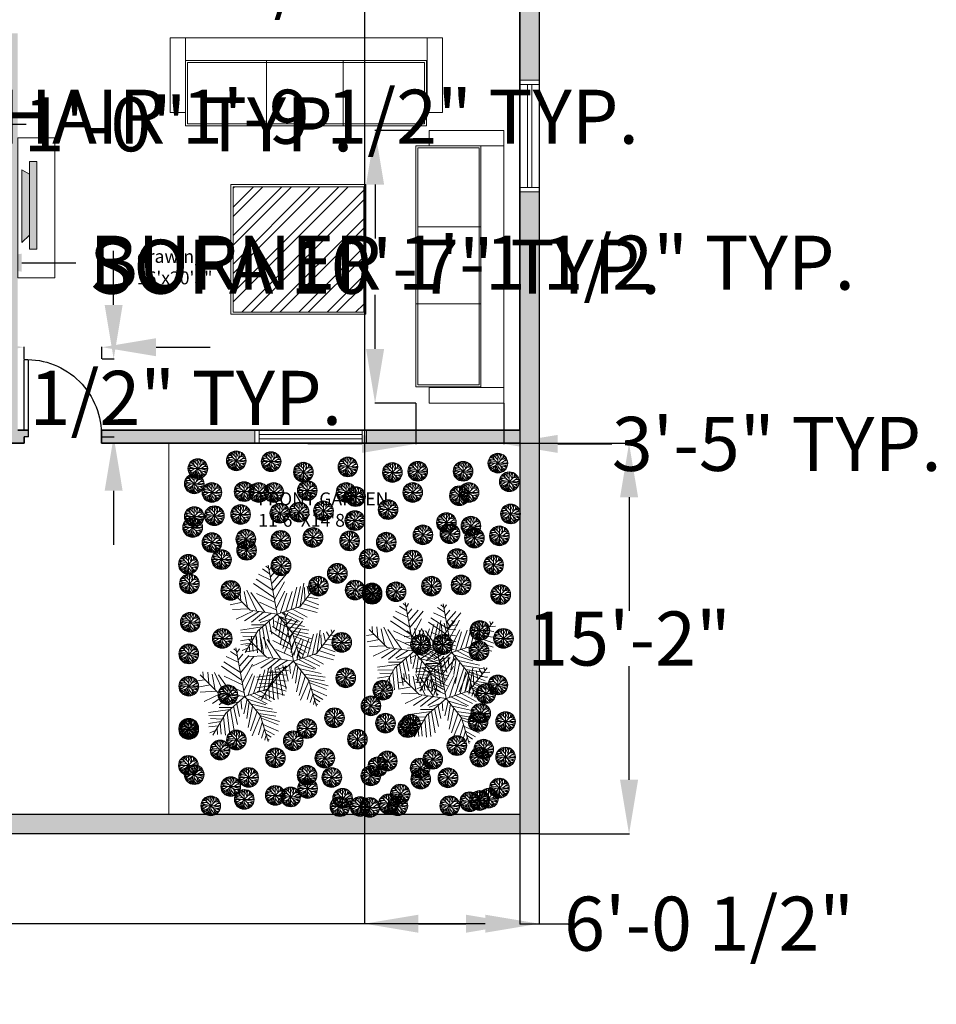
# Model space of a CAD drawing. Units: inches. Extents: x 23 to 3024, y 4 to 1405.
# Tile 4 of 7: x 2558 to 2985, y 497 to 955. Entities that reach past the tile are written whole.
import ezdxf

# ---------------------------------------------------------------- set-up
doc = ezdxf.new("R2010")
doc.units = ezdxf.units.IN
doc.header["$MEASUREMENT"] = 0
for name, color, linetype, lineweight in [('A-ANNO-DIMS', 2, 'Continuous', 18), ('A-DOOR', 4, 'Continuous', 25), ('A-EQPM', 8, 'Continuous', 18), ('A-EQPM-PATT', 7, 'Continuous', 13), ('A-WALL', 7, 'Continuous', 35), ('A-WALL-PATT', 189, 'Continuous', 13), ('C-PROP', 7, 'Continuous', 30), ('L-HRDS', 8, 'Continuous', 18), ('L-PLNT', 114, 'Continuous', 13)]:
    doc.layers.add(name, color=color, linetype=linetype, lineweight=lineweight)
for name, color, linetype, lineweight, true_color in [('A-AREA-IDEN', 30, 'Continuous', 18, 0xf8991e), ('A-FURN', 141, 'Continuous', 18, 0xadddf7), ('A-FURN-PATT', 215, 'Continuous', 13, 0xa953a0), ('A-GLAZ', 30, 'Continuous', 18, 0xf26722)]:
    doc.layers.add(name, color=color, linetype=linetype, lineweight=lineweight, true_color=true_color)
doc.styles.get("Standard").update_dxf_attribs({"font": 'arial.ttf'})
doc.dimstyles.get("Standard").update_dxf_attribs({"dimtxt": 25.18, "dimasz": 25.18, "dimexe": 0.18, "dimexo": 0.0625, "dimgap": 0.09, "dimtad": 0, "dimtih": 1, "dimtoh": 1, "dimdec": 0, "dimrnd": 10, "dimzin": 0, "dimdsep": 46, "dimlunit": 3, "dimtxsty": 'Standard', "dimcen": 0.09, "dimadec": 0, "dimazin": 0, "dimtfac": 1, "dimtdec": 0, "dimtofl": 0, "dimtmove": 0, "dimatfit": 3, "dimfxl": 1, "dimtolj": 1, "dimtzin": 0, "dimarcsym": 0})

# ---------------------------------------------------------------- blocks, each defined once
blk = doc.blocks.new('Tree - deciduous plan')
for p, q in [((2.426, 54.9406), (-1.4472, 59.9056)), ((0, 59.9996), (0, -60)), ((-59.7219, 2.8025), (-12.0106, 12.0565)), ((-32.2571, 20.6333), (-59.1937, 9.348)), ((-58.6656, 12.7336), (-35.9543, 7.5424)), ((-57.081, 17.9248), (-47.0458, 14.7649)), ((-56.0247, 20.859), (-20.8134, 20.859)), ((-54.7923, 24.4702), (-47.75, 21.0847)), ((-54.6162, -24.7335), (-20.2853, 0.0941)), ((-53.2078, 27.4044), (-40.1797, 20.859)), ((-49.8627, 32.8214), (-32.7853, 32.8214)), ((-45.8134, 38.2383), (-40.5318, 33.0471)), ((-43.8768, 36.4326), (-44.405, 40.2696)), ((42, 42), (-42, -42)), ((42, -42), (-42, 42)), ((-40.1797, 44.558), (-36.4825, 43.2038)), ((-37.0107, 47.0408), (-35.25, 35.5298)), ((-32.6092, 50.4264), (-23.2782, 23.5674)), ((-31.2008, 51.1035), (-0.2149, 20.1818)), ((-26.4472, 46.5894), (-26.2712, 53.8116)), ((-22.0458, 42.0753), (-16.5881, 57.6486)), ((-21.1656, 55.8436), (-0.0388, 45.0094)), ((-12.5388, 54.9406), (-7.9613, 59.4546)), ((-12.3627, 32.1443), (-12.5388, 58.7776)), ((-5.3205, 59.6806), (16.5105, 16.7963)), ((0.4894, 48.6208), (3.6584, 59.6806)), ((18.2711, 35.5298), (5.419, 59.6806)), ((9.8203, 51.5549), (12.8133, 58.5516)), ((19.6795, 19.5047), (16.3344, 57.6486)), ((17.0387, 51.1035), (23.2006, 55.1666)), ((17.7429, 43.6552), (25.4894, 54.2636)), ((54.3626, 25.3731), (20.9119, 0.3198)), ((23.3767, 23.3417), (53.3063, 27.4044)), ((29.3626, -6.6771), (59.4682, 7.091)), ((31.6513, 50.8778), (30.2429, 30.5643)), ((31.1232, 42.5267), (35.8767, 48.1693)), ((36.2288, 25.1474), (48.9049, 35.0784)), ((37.1091, 37.1098), (46.6161, 37.5612)), ((38.5175, 13.4107), (58.2359, 13.6364)), ((-60, 0), (60, 0)), ((-59.7219, -4.8714), (-54.2641, -6.6771)), ((-45.2853, -0.1316), (-59.0177, -10.0627)), ((-58.4895, -12.3197), (-36.4825, -11.6426)), ((-57.081, -18.4138), (-45.2853, -17.9624)), ((-52.6797, -18.188), (-55.4966, -22.0251)), ((-53.2078, -27.442), (-16.7641, -16.6081)), ((-38.9472, -29.0219), (-51.4472, -30.6018)), ((-47.2219, -19.3166), (-50.2148, -26.3135)), ((-46.5177, -30.1504), (-49.5106, -33.536)), ((-32.4331, -32.4075), (-48.1021, -35.5674)), ((-43.7008, -34.6645), (-46.6937, -37.373)), ((-35.9543, -22.4765), (-44.0529, -40.5329)), ((-24.6867, -37.8244), (-38.7712, -45.7241)), ((-26.2712, -43.9185), (-34.7219, -48.6583)), ((-19.9331, -20.2194), (-28.5599, -52.721)), ((-14.6515, -36.2445), (-27.6797, -52.9467)), ((-14.6515, -47.3041), (-25.0388, -54.3009)), ((-21.5177, -45.4984), (-19.9331, -56.1065)), ((-14.8275, -15.0282), (-14.6515, -57.6865)), ((-14.6515, -32.1818), (-3.912, -59.4922)), ((-8.4895, -47.5298), (-11.4825, -58.5893)), ((-10.074, -10.0627), (-2.5036, -59.7178)), ((-6.3768, -52.721), (-9.3698, -58.815)), ((-6.2008, -36.2445), (17.919, -57.0094)), ((-0.0388, -19.0909), (25.8415, -53.8495)), ((8.4119, -53.1724), (3.8344, -59.4922)), ((5.9471, -46.6269), (10.5246, -58.5893)), ((9.2922, -9.1598), (59.6443, -2.8401)), ((18.6232, -18.6394), (26.7218, -53.3981)), ((18.7992, -18.6394), (57.3556, -17.2853)), ((22.8485, -36.4702), (35.3485, -48.4326)), ((24.7852, -44.8213), (23.0246, -54.978)), ((26.3697, -18.4138), (58.9401, -9.8369)), ((30.419, -30.1504), (32.3556, -50.0125)), ((31.4753, -31.279), (49.6091, -33.3103)), ((38.1654, -18.188), (52.426, -29.0219)), ((41.5105, -32.6332), (46.088, -38.0501)), ((45.9119, -24.0564), (55.595, -22.2508))]:
    blk.add_line(p, q)
blk.add_circle((0, 0), 60)
blk = doc.blocks.new('*U8')
for p, q in [((-7.288, 39.707), (-21.778, 46.673)), ((-8.737, 47.138), (-17.069, 52.711)), ((-10.186, 53.64), (-13.084, 55.962)), ((0, 0), (-10.5, 57)), ((-9.099, 51.782), (-6.563, 55.962)), ((-7.65, 43.423), (-2.578, 49.46)), ((-5.839, 35.992), (4.667, 48.067)), ((-5.114, 27.632), (10.463, 46.673)), ((-3.665, 19.273), (-27.574, 35.527)), ((-5.114, 28.097), (-24.676, 40.636)), ((-2.941, 16.486), (8.652, 37.85)), ((27, 9), (48, 36)), ((27.127, 9.056), (31.112, 35.992)), ((44.153, 36.456), (45.239, 32.741)), ((-31.5, 4.5), (-52.5, 25.5)), ((-48.585, 21.131), (-49.309, 29.026)), ((-43.513, 28.561), (-42.427, 15.558)), ((-38.442, 26.239), (-34.819, 7.663)), ((-35.544, 28.097), (-24.314, 3.947)), ((-14.533, 2.09), (-30.834, 25.31)), ((-24.314, 23.917), (-2.941, 13.7)), ((-1.129, 6.734), (9.014, 26.704)), ((3.942, 1.625), (11.187, 24.381)), ((10.101, 3.483), (17.708, 26.239)), ((16.259, 5.805), (23.142, 31.348)), ((22.055, 7.198), (27.489, 32.277)), ((31.836, 30.883), (32.561, 16.486)), ((35.096, 32.741), (37.27, 22.524)), ((38.719, 34.134), (41.979, 28.561)), ((40.53, 25.775), (48.862, 24.846)), ((43.791, 29.954), (51.036, 30.883)), ((-47.498, 19.737), (-55.83, 18.344)), ((-40.615, 13.7), (-55.105, 10.913)), ((-20.691, 13.7), (-1.129, 4.876)), ((29.662, 12.307), (48.137, 6.269)), ((33.285, 16.486), (48.862, 10.913)), ((36.183, 19.737), (48.137, 17.88)), ((-33.37, 6.269), (-52.207, 5.34)), ((-28.299, 3.483), (-47.86, -5.805)), ((-21.416, 3.018), (-38.079, -8.128)), ((0, 0), (-31.5, 4.5)), ((-15.982, 2.09), (-30.11, -9.521)), ((0, 0), (-22.5, -19.5)), ((-6.563, 1.161), (-21.416, -8.128)), ((0, 0), (27, 9)), ((0, 0), (18, -22.5)), ((6.478, 1.625), (26.04, -8.592)), ((11.187, 3.483), (30.749, -5.805)), ((18.07, 5.805), (35.096, -3.483)), ((24.229, 7.663), (46.688, 1.625)), ((-6.563, -5.805), (-19.967, -9.985)), ((-13.446, -11.378), (-8.737, -32.741)), ((-9.461, -8.592), (-6.201, -23.453)), ((-4.752, -3.483), (-3.665, -14.629)), ((2.493, -3.019), (-1.491, -20.202)), ((1.769, -2.555), (24.229, -9.521)), ((5.029, -6.27), (2.131, -25.775)), ((9.014, -11.378), (3.58, -35.992)), ((7.565, -9.056), (32.198, -14.629)), ((-17.431, -15.094), (-42.789, -18.809)), ((-24.314, -21.596), (-42.427, -22.06)), ((-22.5, -19.5), (-37.5, -45)), ((-15.257, -12.772), (-30.11, -12.772)), ((-20.691, -18.345), (-17.793, -44.352)), ((-17.069, -15.094), (-12.721, -40.172)), ((14.085, -16.951), (6.478, -40.172)), ((18.07, -22.524), (8.289, -45.745)), ((12.274, -15.094), (36.907, -18.809)), ((16.259, -19.738), (36.183, -22.989)), ((18, -22.5), (27, -52.5)), ((18.433, -22.524), (40.53, -29.026)), ((-28.299, -29.026), (-42.789, -31.348)), ((-30.834, -34.135), (-42.427, -35.528)), ((-26.849, -26.24), (-40.253, -25.775)), ((-29.023, -30.884), (-27.936, -43.887)), ((-25.038, -23.918), (-22.865, -45.281)), ((20.244, -30.419), (15.897, -44.816)), ((19.157, -25.311), (38.719, -33.206)), ((21.331, -32.741), (39.081, -40.636)), ((-34.457, -39.708), (-40.978, -42.494)), ((-32.646, -36.921), (-31.921, -44.352)), ((22.78, -37.85), (19.519, -48.532)), ((22.78, -38.314), (34.372, -44.816)), ((24.591, -45.745), (23.142, -50.854)), ((24.591, -43.423), (30.749, -47.603)), ((26.764, -49.925), (28.213, -50.854))]:
    blk.add_line(p, q)
blk = doc.blocks.new('DOOR-SWING-36IN')
for p, q in [((-1, -1), (-1, 35)), ((1, 2), (1, 35)), ((-1, -1), (1, -1))]:
    blk.add_line(p, q)
blk.add_arc((0, 0), 35.01, 88.3634, 181.6366)
blk = doc.blocks.new('WINDOW-48IN')
for p, q in [((9, 52), (0, 52)), ((9, 50), (0, 50)), ((3.5, 2), (3.5, 50)), ((5.5, 2), (5.5, 50)), ((9, 2), (0, 2)), ((9, 0), (0, 0))]:
    blk.add_line(p, q)
blk = doc.blocks.new('SOFA-THREE-SEAT')
for p, q in [((44.91, 30.29), (44.91, 0.86)), ((80.71, 30.29), (80.71, 0))]:
    blk.add_line(p, q)
for points in [[(7.2, 40.92), (0, 40.92), (0, 6.21), (7.2, 6.21)], [(7.2, 30.29), (119.76, 30.29), (119.76, 40.92), (7.2, 40.92)], [(126.96, 40.92), (119.76, 40.92), (119.76, 6.21), (126.96, 6.21)], [(7.2, 30.29), (119.4, 30.29), (119.4, 0), (7.2, 0)], [(8.06, 29.42), (118.53, 29.42), (118.53, 0.86), (8.06, 0.86)]]:
    blk.add_lwpolyline(points, close=True)
blk = doc.blocks.new('*D21')
at = {"layer": 'A-ANNO-DIMS', "color": 0, "lineweight": -2, "transparency": 16777216}
for p, q in [((2449.18, 913.2), (2449.18, 909.84)), ((2470.74, 913.2), (2470.74, 909.84)), ((2424, 910.02), (2398.82, 910.02)), ((2495.92, 910.02), (2521.1, 910.02))]:
    blk.add_line(p, q, dxfattribs=at)
at = {"layer": 'A-ANNO-DIMS', "color": 0, "transparency": 16777216}
for points in [[(2424, 914.22), (2424, 905.83), (2449.18, 910.02)], [(2495.92, 914.22), (2495.92, 905.83), (2470.74, 910.02)]]:
    blk.add_solid(points, dxfattribs=at)
at = {"layer": 'Defpoints', "color": 0, "transparency": 16777216}
for p in [(2449.18, 913.26), (2470.74, 913.26), (2470.74, 910.02)]:
    blk.add_point(p, dxfattribs=at)
at = {"layer": 'A-ANNO-DIMS', "color": 0, "transparency": 16777216, "insert": (2686.74, 910.02), "char_height": 25.18, "attachment_point": 5}
blk.add_mtext('\\A1;CHAIR 1\'-9 1/2" TYP.', dxfattribs=at)
blk = doc.blocks.new('*D22')
at = {"layer": 'A-ANNO-DIMS', "color": 0, "lineweight": -2, "transparency": 16777216}
for p, q in [((2473.98, 956.88), (2473.98, 982.06)), ((2473.98, 982.06), (2499.16, 982.06)), ((2470.81, 931.7), (2474.16, 931.7)), ((2470.81, 913.26), (2474.16, 913.26)), ((2473.98, 888.08), (2473.98, 862.9))]:
    blk.add_line(p, q, dxfattribs=at)
at = {"layer": 'A-ANNO-DIMS', "color": 0, "transparency": 16777216}
for points in [[(2469.78, 956.88), (2478.17, 956.88), (2473.98, 931.7)], [(2469.78, 888.08), (2478.17, 888.08), (2473.98, 913.26)]]:
    blk.add_solid(points, dxfattribs=at)
at = {"layer": 'Defpoints', "color": 0, "transparency": 16777216}
for p in [(2470.74, 931.7), (2473.98, 931.7), (2470.74, 913.26)]:
    blk.add_point(p, dxfattribs=at)
at = {"layer": 'A-ANNO-DIMS', "color": 0, "transparency": 16777216, "insert": (2604.14, 982.06), "char_height": 25.18, "attachment_point": 5}
blk.add_mtext('\\A1;1\'-6 1/2" TYP.', dxfattribs=at)
blk = doc.blocks.new('*D23')
at = {"layer": 'A-ANNO-DIMS', "color": 0, "lineweight": -2, "transparency": 16777216}
for p, q in [((2560.45, 797.26), (2560.45, 802.82)), ((2596.72, 797.26), (2596.72, 802.82)), ((2535.27, 802.64), (2510.09, 802.64)), ((2621.9, 802.64), (2647.08, 802.64))]:
    blk.add_line(p, q, dxfattribs=at)
at = {"layer": 'A-ANNO-DIMS', "color": 0, "transparency": 16777216}
for points in [[(2535.27, 806.84), (2535.27, 798.45), (2560.45, 802.64)], [(2621.9, 806.84), (2621.9, 798.45), (2596.72, 802.64)]]:
    blk.add_solid(points, dxfattribs=at)
at = {"layer": 'Defpoints', "color": 0, "transparency": 16777216}
for p in [(2560.45, 802.64), (2560.45, 797.2), (2596.72, 797.2)]:
    blk.add_point(p, dxfattribs=at)
at = {"layer": 'A-ANNO-DIMS', "color": 0, "transparency": 16777216, "insert": (2346.9, 802.64), "char_height": 25.18, "attachment_point": 5}
blk.add_mtext('\\A1;DOOR 3\'-0 1/2" TYP.', dxfattribs=at)
blk = doc.blocks.new('*D24')
at = {"layer": 'A-ANNO-DIMS', "color": 0, "lineweight": -2, "transparency": 16777216}
for p, q in [((2602.17, 822.38), (2602.17, 847.56)), ((2596.79, 797.2), (2602.35, 797.2)), ((2596.79, 760.93), (2602.35, 760.93)), ((2602.17, 735.75), (2602.17, 710.57))]:
    blk.add_line(p, q, dxfattribs=at)
at = {"layer": 'A-ANNO-DIMS', "color": 0, "transparency": 16777216}
for points in [[(2597.97, 822.38), (2606.36, 822.38), (2602.17, 797.2)], [(2597.97, 735.75), (2606.36, 735.75), (2602.17, 760.93)]]:
    blk.add_solid(points, dxfattribs=at)
at = {"layer": 'Defpoints', "color": 0, "transparency": 16777216}
for p in [(2596.72, 797.2), (2602.17, 797.2), (2596.72, 760.93)]:
    blk.add_point(p, dxfattribs=at)
at = {"layer": 'A-ANNO-DIMS', "color": 0, "transparency": 16777216, "insert": (2602.17, 779.06), "char_height": 25.18, "attachment_point": 5}
blk.add_mtext('\\A1;3\'-0 1/2" TYP.', dxfattribs=at)
blk = doc.blocks.new('*D31')
at = {"layer": 'A-ANNO-DIMS', "color": 0, "lineweight": -2, "transparency": 16777216}
for p, q in [((2742.95, 903.61), (2723.79, 903.61)), ((2723.97, 878.43), (2723.97, 853.25)), ((2723.97, 801.83), (2723.97, 827.01)), ((2742.95, 776.65), (2723.79, 776.65))]:
    blk.add_line(p, q, dxfattribs=at)
at = {"layer": 'A-ANNO-DIMS', "color": 0, "transparency": 16777216}
for points in [[(2719.77, 878.43), (2728.17, 878.43), (2723.97, 903.61)], [(2719.77, 801.83), (2728.17, 801.83), (2723.97, 776.65)]]:
    blk.add_solid(points, dxfattribs=at)
at = {"layer": 'Defpoints', "color": 0, "transparency": 16777216}
for p in [(2743.01, 903.61), (2723.97, 776.65), (2743.01, 776.65)]:
    blk.add_point(p, dxfattribs=at)
at = {"layer": 'A-ANNO-DIMS', "color": 0, "transparency": 16777216, "insert": (2723.97, 840.13), "char_height": 25.18, "attachment_point": 5}
blk.add_mtext('\\A1;SOFA 10\'-7" TYP.', dxfattribs=at)
blk = doc.blocks.new('*D32')
at = {"layer": 'A-ANNO-DIMS', "color": 0, "lineweight": -2, "transparency": 16777216}
for p, q in [((2743.01, 776.59), (2743.01, 757.43)), ((2783.93, 776.59), (2783.93, 757.43)), ((2717.83, 757.61), (2692.65, 757.61)), ((2809.11, 757.61), (2834.29, 757.61))]:
    blk.add_line(p, q, dxfattribs=at)
at = {"layer": 'A-ANNO-DIMS', "color": 0, "transparency": 16777216}
for points in [[(2717.83, 761.8), (2717.83, 753.41), (2743.01, 757.61)], [(2809.11, 761.8), (2809.11, 753.41), (2783.93, 757.61)]]:
    blk.add_solid(points, dxfattribs=at)
at = {"layer": 'Defpoints', "color": 0, "transparency": 16777216}
for p in [(2743.01, 776.65), (2783.93, 776.65), (2783.93, 757.61)]:
    blk.add_point(p, dxfattribs=at)
at = {"layer": 'A-ANNO-DIMS', "color": 0, "transparency": 16777216, "insert": (2911.12, 757.61), "char_height": 25.18, "attachment_point": 5}
blk.add_mtext('\\A1;3\'-5" TYP.', dxfattribs=at)
blk = doc.blocks.new('*D33')
at = {"layer": 'A-ANNO-DIMS', "color": 0, "lineweight": -2, "transparency": 16777216}
for p, q in [((2495.35, 842.02), (2470.17, 842.02)), ((2520.53, 844), (2520.53, 841.84)), ((2534.13, 844), (2534.13, 841.84)), ((2559.31, 842.02), (2584.49, 842.02))]:
    blk.add_line(p, q, dxfattribs=at)
at = {"layer": 'A-ANNO-DIMS', "color": 0, "transparency": 16777216}
for points in [[(2495.35, 846.22), (2495.35, 837.83), (2520.53, 842.02)], [(2559.31, 846.22), (2559.31, 837.83), (2534.13, 842.02)]]:
    blk.add_solid(points, dxfattribs=at)
at = {"layer": 'Defpoints', "color": 0, "transparency": 16777216}
for p in [(2520.53, 844.06), (2534.13, 844.06), (2534.13, 842.02)]:
    blk.add_point(p, dxfattribs=at)
at = {"layer": 'A-ANNO-DIMS', "color": 0, "transparency": 16777216, "insert": (2769.25, 842.02), "char_height": 25.18, "attachment_point": 5}
blk.add_mtext('\\A1;BURNER 1\'-1 1/2" TYP.', dxfattribs=at)
blk = doc.blocks.new('*D34')
at = {"layer": 'A-ANNO-DIMS', "color": 0, "lineweight": -2, "transparency": 16777216}
for p, q in [((2536.16, 881.33), (2536.16, 906.51)), ((2536.16, 906.51), (2561.34, 906.51)), ((2534.19, 856.15), (2536.34, 856.15)), ((2534.19, 844.06), (2536.34, 844.06)), ((2536.16, 818.88), (2536.16, 793.7))]:
    blk.add_line(p, q, dxfattribs=at)
at = {"layer": 'A-ANNO-DIMS', "color": 0, "transparency": 16777216}
for points in [[(2531.97, 881.33), (2540.36, 881.33), (2536.16, 856.15)], [(2531.97, 818.88), (2540.36, 818.88), (2536.16, 844.06)]]:
    blk.add_solid(points, dxfattribs=at)
at = {"layer": 'Defpoints', "color": 0, "transparency": 16777216}
for p in [(2534.13, 856.15), (2536.16, 856.15), (2534.13, 844.06)]:
    blk.add_point(p, dxfattribs=at)
at = {"layer": 'A-ANNO-DIMS', "color": 0, "transparency": 16777216, "insert": (2636.99, 906.51), "char_height": 25.18, "attachment_point": 5}
blk.add_mtext('\\A1;1\'-0" TYP.', dxfattribs=at)
blk = doc.blocks.new('*D35')
at = {"layer": 'A-ANNO-DIMS', "color": 0, "lineweight": -2, "transparency": 16777216}
for p, q in [((2272.06, 973.9), (2246.88, 973.9)), ((2297.24, 975.85), (2297.24, 973.72)), ((2310.67, 975.85), (2310.67, 973.72)), ((2335.85, 973.9), (2361.03, 973.9))]:
    blk.add_line(p, q, dxfattribs=at)
at = {"layer": 'A-ANNO-DIMS', "color": 0, "transparency": 16777216}
for points in [[(2272.06, 978.09), (2272.06, 969.7), (2297.24, 973.9)], [(2335.85, 978.09), (2335.85, 969.7), (2310.67, 973.9)]]:
    blk.add_solid(points, dxfattribs=at)
at = {"layer": 'Defpoints', "color": 0, "transparency": 16777216}
for p in [(2297.24, 975.91), (2310.67, 975.91), (2310.67, 973.9)]:
    blk.add_point(p, dxfattribs=at)
at = {"layer": 'A-ANNO-DIMS', "color": 0, "transparency": 16777216, "insert": (2585.8, 973.9), "char_height": 25.18, "attachment_point": 5}
blk.add_mtext('\\A1;NIGHTSTAND 1\'-1 1/2" TYP.', dxfattribs=at)
blk = doc.blocks.new('*D41')
at = {"layer": 'A-ANNO-DIMS', "color": 0, "lineweight": -2, "transparency": 16777216}
for p, q in [((2160.45, 575.86), (2160.45, 533.9)), ((2800.45, 575.86), (2800.45, 533.9)), ((2185.63, 534.08), (2437.11, 534.08)), ((2775.27, 534.08), (2523.79, 534.08))]:
    blk.add_line(p, q, dxfattribs=at)
at = {"layer": 'A-ANNO-DIMS', "color": 0, "transparency": 16777216}
for points in [[(2185.63, 538.27), (2185.63, 529.88), (2160.45, 534.08)], [(2775.27, 538.27), (2775.27, 529.88), (2800.45, 534.08)]]:
    blk.add_solid(points, dxfattribs=at)
at = {"layer": 'Defpoints', "color": 0, "transparency": 16777216}
for p in [(2160.45, 575.93), (2800.45, 575.93), (2800.45, 534.08)]:
    blk.add_point(p, dxfattribs=at)
at = {"layer": 'A-ANNO-DIMS', "color": 0, "transparency": 16777216, "insert": (2480.45, 534.08), "char_height": 25.18, "attachment_point": 5}
blk.add_mtext('\\A1;53\'-4"', dxfattribs=at)
blk = doc.blocks.new('*D42')
at = {"layer": 'A-ANNO-DIMS', "color": 0, "lineweight": -2, "transparency": 16777216}
for p, q in [((2791.51, 757.93), (2842.48, 757.93)), ((2842.3, 732.75), (2842.3, 679.87)), ((2842.3, 601.11), (2842.3, 653.98)), ((2800.51, 575.93), (2842.48, 575.93))]:
    blk.add_line(p, q, dxfattribs=at)
at = {"layer": 'A-ANNO-DIMS', "color": 0, "transparency": 16777216}
for points in [[(2838.1, 732.75), (2846.5, 732.75), (2842.3, 757.93)], [(2838.1, 601.11), (2846.5, 601.11), (2842.3, 575.93)]]:
    blk.add_solid(points, dxfattribs=at)
at = {"layer": 'Defpoints', "color": 0, "transparency": 16777216}
for p in [(2791.45, 757.93), (2842.3, 757.93), (2800.45, 575.93)]:
    blk.add_point(p, dxfattribs=at)
at = {"layer": 'A-ANNO-DIMS', "color": 0, "transparency": 16777216, "insert": (2842.3, 666.93), "char_height": 25.18, "attachment_point": 5}
blk.add_mtext('\\A1;15\'-2"', dxfattribs=at)
blk = doc.blocks.new('*D45')
at = {"layer": 'A-ANNO-DIMS', "color": 0, "lineweight": -2, "transparency": 16777216}
for p, q in [((2719, 988.72), (2719, 533.9)), ((2791.45, 988.72), (2791.45, 533.9)), ((2744.18, 534.08), (2766.27, 534.08)), ((2791.45, 534.08), (2816.63, 534.08))]:
    blk.add_line(p, q, dxfattribs=at)
at = {"layer": 'A-ANNO-DIMS', "color": 0, "transparency": 16777216}
for points in [[(2744.18, 538.27), (2744.18, 529.88), (2719, 534.08)], [(2766.27, 538.27), (2766.27, 529.88), (2791.45, 534.08)]]:
    blk.add_solid(points, dxfattribs=at)
at = {"layer": 'Defpoints', "color": 0, "transparency": 16777216}
for p in [(2719, 988.78), (2791.45, 988.78), (2791.45, 534.08)]:
    blk.add_point(p, dxfattribs=at)
at = {"layer": 'A-ANNO-DIMS', "color": 0, "transparency": 16777216, "insert": (2879.59, 534.08), "char_height": 25.18, "attachment_point": 5}
blk.add_mtext('\\A1;6\'-0 1/2"', dxfattribs=at)

msp = doc.modelspace()

# ---------------------------------------------------------------- hatches: boundary and pattern name
at = {"layer": 'A-EQPM-PATT'}
h = msp.add_hatch(color=256, dxfattribs=at)
h.dxf.hatch_style = 1
h.paths.add_polyline_path([(2566.39, 889.19), (2562.89, 889.19), (2562.89, 848.35), (2566.39, 848.35)])
h.paths.add_polyline_path([(2562.89, 883.28), (2559.32, 885.34), (2559.32, 851.44), (2562.89, 854.81)])
h.paths.add_polyline_path([(2370.36, 1159.16), (2369.43, 1157.81), (2369.43, 1135.58), (2370.36, 1134.43)])
h.paths.add_polyline_path([(2369.43, 1162.31), (2367.73, 1162.31), (2367.73, 1131.3), (2369.43, 1131.3)])
h.paths.add_polyline_path([(2381.34, 1160.62), (2379.7, 1162.16), (2380.08, 1134.79), (2381.34, 1136.43)])
h.paths.add_polyline_path([(2383.55, 1164.18), (2381.34, 1164.18), (2381.34, 1130.16), (2383.55, 1130.16)])
at = {"layer": 'A-FURN-PATT'}
h = msp.add_hatch(dxfattribs=at)
h.set_pattern_fill('ANSI32', color=256, scale=25)
h.paths.add_polyline_path([(2718.66, 877.42), (2657.77, 877.42), (2657.77, 818.97), (2718.66, 818.97)])
at = {"layer": 'A-WALL-PATT'}
h = msp.add_hatch(color=256, dxfattribs=at)
h.dxf.hatch_style = 1
h.paths.add_polyline_path([(2209.45, 1233.93), (2200.45, 1233.93), (2200.45, 1160.43), (2209.45, 1160.43), (2209.45, 1167.77), (2209.45, 1202.93), (2306.45, 1202.93), (2306.45, 1208.93), (2300.45, 1208.93), (2209.45, 1208.93)], flags=17)
h.paths.add_polyline_path([(2800.45, 1295.93), (2200.45, 1295.93), (2160.45, 1295.93), (2160.45, 575.93), (2200.45, 575.93), (2228.06, 575.93), (2228.06, 584.93), (2209.45, 584.93), (2209.45, 856.93), (2200.45, 856.93), (2200.45, 581.93), (2166.45, 581.93), (2166.45, 1289.93), (2200.45, 1289.93), (2200.45, 1261.93), (2209.45, 1261.93), (2209.45, 1286.93), (2244.45, 1286.93), (2300.45, 1286.93), (2300.45, 1241.93), (2301.45, 1241.93, -0.017236), (2303.45, 1241.93), (2306.45, 1241.93), (2306.45, 1286.93), (2548.45, 1286.93), (2548.45, 1261.93), (2557.45, 1261.93), (2557.45, 1286.93), (2791.45, 1286.93), (2791.45, 1140.93), (2613.74, 1140.93), (2613.74, 1134.93), (2791.45, 1134.93), (2791.45, 927.1), (2800.45, 927.1)])
h.paths.add_polyline_path([(2166.06, 1284.53), (2166.03, 1284.87), (2166.29, 1284.91), (2166.32, 1284.58)], flags=16)
h.paths.add_polyline_path([(2557.45, 1233.93), (2548.45, 1233.93), (2548.45, 1208.93), (2514.78, 1208.93), (2457.45, 1208.93), (2451.45, 1208.93), (2451.45, 1202.93), (2548.45, 1202.93), (2557.45, 1202.93)], flags=17)
h.paths.add_polyline_path([(2457.45, 1286.93), (2451.45, 1286.93), (2451.45, 1241.93), (2454.45, 1241.93, -0.017236), (2456.45, 1241.93), (2457.45, 1241.93)], flags=17)
h.paths.add_polyline_path([(2419.96, 1208.93), (2378.45, 1208.93), (2378.45, 1286.93), (2372.45, 1286.93), (2372.45, 1208.93), (2352.45, 1208.93), (2352.45, 1202.93), (2419.96, 1202.93)], flags=17)
h.paths.add_polyline_path([(2557.45, 1134.93), (2563.84, 1134.93), (2563.84, 1140.93), (2557.45, 1140.93), (2557.45, 1149.12), (2548.45, 1149.12), (2548.45, 1103.07), (2548.45, 1065.93), (2416.45, 1065.93), (2416.45, 1064.93, -0.014283), (2416.45, 1062.93), (2416.45, 1059.93), (2548.45, 1059.93), (2548.45, 1025.12), (2557.45, 1025.12)], flags=17)
h.paths.add_polyline_path([(2332.45, 1062.93, -0.014283), (2332.45, 1064.93), (2332.45, 1065.93), (2209.45, 1065.93), (2209.45, 1108.43), (2200.45, 1108.43), (2200.45, 1042.43), (2209.45, 1042.43), (2209.45, 1059.93), (2332.45, 1059.93)], flags=17)
h.paths.add_polyline_path([(2332.45, 996.93), (2209.45, 996.93), (2209.45, 1014.43), (2200.45, 1014.43), (2200.45, 952.93), (2209.45, 952.93), (2209.45, 990.93), (2332.45, 990.93), (2332.45, 991.93, -0.014283), (2332.45, 993.93)], flags=17)
h.paths.add_polyline_path([(2209.45, 900.93), (2200.45, 900.93), (2200.45, 856.93), (2209.45, 856.93), (2255.95, 856.93), (2255.95, 862.93), (2209.45, 862.93)], flags=17)
h.paths.add_polyline_path([(2377.45, 823.93), (2374.45, 823.93, -0.017236), (2372.45, 823.93), (2371.45, 823.93), (2371.45, 763.93), (2312.45, 763.93), (2312.45, 791.27), (2312.45, 796.43), (2306.45, 796.43), (2306.45, 757.93), (2436.95, 757.93), (2436.95, 763.93), (2377.45, 763.93)], flags=17)
h.paths.add_polyline_path([(2557.45, 948.81), (2548.45, 948.81), (2548.45, 763.93), (2488.95, 763.93), (2488.95, 757.93), (2560.45, 757.93), (2560.45, 760.93), (2562.45, 760.93), (2562.45, 763.93), (2557.45, 763.93)], flags=17)
h.paths.add_polyline_path([(2377.45, 990.93), (2371.45, 990.93), (2371.45, 862.93), (2306.45, 862.93), (2306.45, 856.93), (2306.45, 824.43), (2312.45, 824.43), (2312.45, 856.93), (2371.45, 856.93), (2377.45, 856.93)], flags=17)
h.paths.add_polyline_path([(2800.45, 875.1), (2791.45, 875.1), (2791.45, 763.93), (2719.93, 763.93), (2719.93, 757.93), (2791.45, 757.93), (2791.45, 584.93), (2338.88, 584.93), (2338.88, 575.93), (2800.45, 575.93)], flags=17)
h.paths.add_polyline_path([(2667.93, 763.93), (2596.45, 763.93), (2596.45, 762.93, -0.014283), (2596.45, 760.93), (2596.45, 757.93), (2667.93, 757.93)], flags=16)

# ---------------------------------------------------------------- linework, layer by layer
at = {"layer": 'A-EQPM'}
for p, q in [((2562.89, 883.28), (2559.32, 885.34)), ((2559.32, 885.34), (2559.32, 851.44)), ((2559.32, 851.44), (2562.89, 854.81))]:
    msp.add_line(p, q, dxfattribs=at)
for points in [[(2557.45, 900.13), (2574.69, 900.13), (2574.69, 834.99), (2557.45, 834.99)], [(2562.89, 889.19), (2566.39, 889.19), (2566.39, 848.35), (2562.89, 848.35)]]:
    msp.add_lwpolyline(points, close=True, dxfattribs=at)
at = {"layer": 'A-FURN'}
for points in [[(2656.77, 878.42), (2719.66, 878.42), (2719.66, 817.97), (2656.77, 817.97)], [(2657.77, 877.42), (2718.66, 877.42), (2718.66, 818.97), (2657.77, 818.97)]]:
    msp.add_lwpolyline(points, close=True, dxfattribs=at)
at = {"layer": 'A-GLAZ'}
for p, q in [((2667.93, 763.93), (2667.93, 757.93)), ((2669.93, 763.93), (2669.93, 757.93)), ((2669.93, 761.93), (2717.93, 761.93)), ((2717.93, 763.93), (2717.93, 757.93)), ((2719.93, 763.93), (2719.93, 757.93)), ((2669.93, 759.93), (2717.93, 759.93))]:
    msp.add_line(p, q, dxfattribs=at)
at = {"layer": 'A-WALL'}
for p, q in [((2791.45, 1134.93), (2791.45, 763.93)), ((2557.45, 763.93), (2562.45, 763.93)), ((2596.41, 763.93), (2791.45, 763.93)), ((2596.45, 763.93), (2596.45, 757.93)), ((2306.45, 757.93), (2560.45, 757.93)), ((2560.45, 760.93), (2560.45, 757.93)), ((2596.45, 757.93), (2791.45, 757.93))]:
    msp.add_line(p, q, dxfattribs=at)
at = {"layer": 'C-PROP'}
for p, q in [((2800.45, 1295.93), (2800.45, 575.93)), ((2791.45, 757.93), (2791.45, 584.93)), ((2791.45, 584.93), (2338.88, 584.93)), ((2800.45, 575.93), (2338.88, 575.93))]:
    msp.add_line(p, q, dxfattribs=at)
at = {"layer": 'L-HRDS'}
msp.add_line((2627.88, 757.93), (2627.88, 584.93), dxfattribs=at)

# ---------------------------------------------------------------- block references
at = {"layer": 'A-DOOR', "extrusion": (0, 0, -1), "zscale": -1}
msp.add_blockref('DOOR-SWING-36IN', (-2561.45, 761.93), dxfattribs=at)
at = {"layer": 'A-FURN'}
msp.add_blockref('SOFA-THREE-SEAT', (2628.45, 905.85), dxfattribs=at)
at = {"layer": 'A-FURN', "rotation": 270.0000000000003}
msp.add_blockref('SOFA-THREE-SEAT', (2743.01, 903.61), dxfattribs=at)
at = {"layer": 'A-GLAZ'}
msp.add_blockref('WINDOW-48IN', (2791.45, 875.1), dxfattribs=at)
at = {"layer": 'L-PLNT'}
for name, p, xscale, yscale, zscale in [('Tree - deciduous plan', (2659.27, 749.73), 0.0767429263113536, 0.0767429263113536, 0.0767429263113536), ('Tree - deciduous plan', (2675.53, 749.33), 0.0767429263113536, 0.0767429263113536, 0.0767429263113536), ('Tree - deciduous plan', (2781.18, 748.62), 0.0767429263113536, 0.0767429263113536, 0.0767429263113536), ('Tree - deciduous plan', (2641.39, 746.08), 0.0767429263113536, 0.0767429263113536, 0.0767429263113536), ('Tree - deciduous plan', (2690.57, 744.46), 0.0767429263113536, 0.0767429263113536, 0.0767429263113536), ('Tree - deciduous plan', (2711.3, 746.89), 0.0767429263113536, 0.0767429263113536, 0.0767429263113536), ('Tree - deciduous plan', (2732.03, 744.29), 0.0767429263113536, 0.0767429263113536, 0.0767429263113536), ('Tree - deciduous plan', (2743.82, 744.86), 0.0767429263113536, 0.0767429263113536, 0.0767429263113536), ('Tree - deciduous plan', (2764.95, 744.86), 0.0767429263113536, 0.0767429263113536, 0.0767429263113536), ('Tree - deciduous plan', (2639.7, 739.02), 0.0767429263113536, 0.0767429263113536, 0.0767429263113536), ('Tree - deciduous plan', (2786.5, 739.99), 0.0767429263113536, 0.0767429263113536, 0.0767429263113536), ('Tree - deciduous plan', (2647.95, 734.97), 0.0767429263113536, 0.0767429263113536, 0.0767429263113536), ('Tree - deciduous plan', (2662.94, 735.36), 0.0767429263113536, 0.0767429263113536, 0.0767429263113536), ('Tree - deciduous plan', (2669.78, 734.97), 0.0767429263113536, 0.0767429263113536, 0.0767429263113536), ('Tree - deciduous plan', (2676.78, 734.97), 0.0767429263113536, 0.0767429263113536, 0.0767429263113536), ('Tree - deciduous plan', (2692.36, 735.83), 0.0767429263113536, 0.0767429263113536, 0.0767429263113536), ('Tree - deciduous plan', (2710.46, 734.97), 0.0767429263113536, 0.0767429263113536, 0.0767429263113536), ('Tree - deciduous plan', (2741.51, 734.97), 0.0767429263113536, 0.0767429263113536, 0.0767429263113536), ('Tree - deciduous plan', (2767.72, 734.97), 0.0767429263113536, 0.0767429263113536, 0.0767429263113536), ('Tree - deciduous plan', (2714.86, 733.07), 0.0767429263113536, 0.0767429263113536, 0.0767429263113536), ('Tree - deciduous plan', (2763.23, 733.45), 0.0767429263113536, 0.0767429263113536, 0.0767429263113536), ('Tree - deciduous plan', (2679.6, 725.29), 0.0767429263113536, 0.0767429263113536, 0.0767429263113536), ('Tree - deciduous plan', (2688.54, 725.86), 0.0767429263113536, 0.0767429263113536, 0.0767429263113536), ('Tree - deciduous plan', (2699.92, 726.43), 0.0767429263113536, 0.0767429263113536, 0.0767429263113536), ('Tree - deciduous plan', (2730, 727), 0.0767429263113536, 0.0767429263113536, 0.0767429263113536), ('Tree - deciduous plan', (2787.07, 724.96), 0.0767429263113536, 0.0767429263113536, 0.0767429263113536), ('Tree - deciduous plan', (2639.7, 723.75), 0.0767429263113536, 0.0767429263113536, 0.0767429263113536), ('Tree - deciduous plan', (2649.11, 724.15), 0.0767429263113536, 0.0767429263113536, 0.0767429263113536), ('Tree - deciduous plan', (2661.3, 724.72), 0.0767429263113536, 0.0767429263113536, 0.0767429263113536), ('Tree - deciduous plan', (2714.53, 721.86), 0.0767429263113536, 0.0767429263113536, 0.0767429263113536), ('Tree - deciduous plan', (2757.18, 720.96), 0.0767429263113536, 0.0767429263113536, 0.0767429263113536), ('Tree - deciduous plan', (2638.98, 718.67), 0.0767429263113536, 0.0767429263113536, 0.0767429263113536), ('Tree - deciduous plan', (2758.88, 715.74), 0.0767429263113536, 0.0767429263113536, 0.0767429263113536), ('Tree - deciduous plan', (2768.61, 719.29), 0.0767429263113536, 0.0767429263113536, 0.0767429263113536), ('Tree - deciduous plan', (2647.95, 711.63), 0.0767429263113536, 0.0767429263113536, 0.0767429263113536), ('Tree - deciduous plan', (2663.74, 713.2), 0.0767429263113536, 0.0767429263113536, 0.0767429263113536), ('Tree - deciduous plan', (2680, 712.63), 0.0767429263113536, 0.0767429263113536, 0.0767429263113536), ('Tree - deciduous plan', (2695.04, 714), 0.0767429263113536, 0.0767429263113536, 0.0767429263113536), ('Tree - deciduous plan', (2712.11, 712.38), 0.0767429263113536, 0.0767429263113536, 0.0767429263113536), ('Tree - deciduous plan', (2729.18, 711.81), 0.0767429263113536, 0.0767429263113536, 0.0767429263113536), ('Tree - deciduous plan', (2746.26, 715.23), 0.0767429263113536, 0.0767429263113536, 0.0767429263113536), ('Tree - deciduous plan', (2770.25, 713.77), 0.0767429263113536, 0.0767429263113536, 0.0767429263113536), ('Tree - deciduous plan', (2781.87, 714.78), 0.0767429263113536, 0.0767429263113536, 0.0767429263113536), ('Tree - deciduous plan', (2664.1, 708.04), 0.0767429263113536, 0.0767429263113536, 0.0767429263113536), ('Tree - deciduous plan', (2652.42, 703.72), 0.0767429263113536, 0.0767429263113536, 0.0767429263113536), ('Tree - deciduous plan', (2721.19, 704.07), 0.0767429263113536, 0.0767429263113536, 0.0767429263113536), ('Tree - deciduous plan', (2741.42, 703.5), 0.0767429263113536, 0.0767429263113536, 0.0767429263113536), ('Tree - deciduous plan', (2762.17, 704.17), 0.0767429263113536, 0.0767429263113536, 0.0767429263113536), ('Tree - deciduous plan', (2636.99, 701.51), 0.0767429263113536, 0.0767429263113536, 0.0767429263113536), ('Tree - deciduous plan', (2680.14, 700.82), 0.0767429263113536, 0.0767429263113536, 0.0767429263113536), ('Tree - deciduous plan', (2706.38, 697.3), 0.0767429263113536, 0.0767429263113536, 0.0767429263113536), ('Tree - deciduous plan', (2779.19, 701.2), 0.0767429263113536, 0.0767429263113536, 0.0767429263113536), ('*U8', (2678.33, 678.34), 0.3984345914112191, 0.3984345914112191, 0.3984345914112191), ('Tree - deciduous plan', (2637.45, 692.43), 0.0767429263113536, 0.0767429263113536, 0.0767429263113536), ('Tree - deciduous plan', (2656.73, 689.36), 0.0767429263113536, 0.0767429263113536, 0.0767429263113536), ('Tree - deciduous plan', (2697.55, 691.34), 0.0767429263113536, 0.0767429263113536, 0.0767429263113536), ('Tree - deciduous plan', (2714.67, 689.51), 0.0767429263113536, 0.0767429263113536, 0.0767429263113536), ('Tree - deciduous plan', (2722.57, 688.14), 0.0767429263113536, 0.0767429263113536, 0.0767429263113536), ('Tree - deciduous plan', (2733.76, 688.71), 0.0767429263113536, 0.0767429263113536, 0.0767429263113536), ('Tree - deciduous plan', (2750.22, 691.34), 0.0767429263113536, 0.0767429263113536, 0.0767429263113536), ('Tree - deciduous plan', (2764.03, 691.88), 0.0767429263113536, 0.0767429263113536, 0.0767429263113536), ('Tree - deciduous plan', (2722.57, 687.57), 0.0767429263113536, 0.0767429263113536, 0.0767429263113536), ('Tree - deciduous plan', (2782.48, 687.39), 0.0767429263113536, 0.0767429263113536, 0.0767429263113536), ('*U8', (2742.19, 661.02), 0.3984345914112191, 0.3984345914112191, 0.3984345914112191), ('Tree - deciduous plan', (2637.86, 674.53), 0.0767429263113536, 0.0767429263113536, 0.0767429263113536), ('*U8', (2685.98, 656.41), 0.3984345914112191, 0.3984345914112191, 0.3984345914112191), ('*U8', (2759.8, 660.38), 0.3984345914112191, 0.3984345914112191, 0.3984345914112191), ('Tree - deciduous plan', (2772.79, 670.67), 0.0767429263113536, 0.0767429263113536, 0.0767429263113536), ('Tree - deciduous plan', (2652.78, 667.01), 0.0767429263113536, 0.0767429263113536, 0.0767429263113536), ('Tree - deciduous plan', (2708.42, 665.14), 0.0767429263113536, 0.0767429263113536, 0.0767429263113536), ('Tree - deciduous plan', (2783.79, 667.01), 0.0767429263113536, 0.0767429263113536, 0.0767429263113536), ('Tree - deciduous plan', (2745.13, 664.08), 0.0767429263113536, 0.0767429263113536, 0.0767429263113536), ('Tree - deciduous plan', (2755.45, 664.08), 0.0767429263113536, 0.0767429263113536, 0.0767429263113536), ('Tree - deciduous plan', (2772.38, 661.19), 0.0767429263113536, 0.0767429263113536, 0.0767429263113536), ('Tree - deciduous plan', (2637.16, 659.75), 0.0767429263113536, 0.0767429263113536, 0.0767429263113536), ('*U8', (2663.34, 639.89), 0.3984345914112191, 0.3984345914112191, 0.3984345914112191), ('*U8', (2757.06, 639), 0.3984345914112191, 0.3984345914112191, 0.3984345914112191), ('Tree - deciduous plan', (2710.28, 648.61), 0.0767429263113536, 0.0767429263113536, 0.0767429263113536), ('Tree - deciduous plan', (2637.16, 644.72), 0.0767429263113536, 0.0767429263113536, 0.0767429263113536), ('Tree - deciduous plan', (2727.58, 642.88), 0.0767429263113536, 0.0767429263113536, 0.0767429263113536), ('Tree - deciduous plan', (2781.16, 645.31), 0.0767429263113536, 0.0767429263113536, 0.0767429263113536), ('Tree - deciduous plan', (2655.42, 640.71), 0.0767429263113536, 0.0767429263113536, 0.0767429263113536), ('Tree - deciduous plan', (2775.59, 641.26), 0.0767429263113536, 0.0767429263113536, 0.0767429263113536), ('Tree - deciduous plan', (2722.02, 635.56), 0.0767429263113536, 0.0767429263113536, 0.0767429263113536), ('Tree - deciduous plan', (2705.04, 630.05), 0.0767429263113536, 0.0767429263113536, 0.0767429263113536), ('Tree - deciduous plan', (2773.2, 632.07), 0.0767429263113536, 0.0767429263113536, 0.0767429263113536), ('Tree - deciduous plan', (2637.16, 625.11), 0.0767429263113536, 0.0767429263113536, 0.0767429263113536), ('Tree - deciduous plan', (2637.16, 624.54), 0.0767429263113536, 0.0767429263113536, 0.0767429263113536), ('Tree - deciduous plan', (2692.21, 624.99), 0.0767429263113536, 0.0767429263113536, 0.0767429263113536), ('Tree - deciduous plan', (2728.82, 627.52), 0.0767429263113536, 0.0767429263113536, 0.0767429263113536), ('Tree - deciduous plan', (2739.19, 625.44), 0.0767429263113536, 0.0767429263113536, 0.0767429263113536), ('Tree - deciduous plan', (2740.49, 627.06), 0.0767429263113536, 0.0767429263113536, 0.0767429263113536), ('Tree - deciduous plan', (2771.94, 628.21), 0.0767429263113536, 0.0767429263113536, 0.0767429263113536), ('Tree - deciduous plan', (2784.76, 628.21), 0.0767429263113536, 0.0767429263113536, 0.0767429263113536), ('Tree - deciduous plan', (2659.37, 619.66), 0.0767429263113536, 0.0767429263113536, 0.0767429263113536), ('Tree - deciduous plan', (2685.87, 619.33), 0.0767429263113536, 0.0767429263113536, 0.0767429263113536), ('Tree - deciduous plan', (2715.73, 620), 0.0767429263113536, 0.0767429263113536, 0.0767429263113536), ('Tree - deciduous plan', (2651.72, 615), 0.0767429263113536, 0.0767429263113536, 0.0767429263113536), ('Tree - deciduous plan', (2762.07, 617.03), 0.0767429263113536, 0.0767429263113536, 0.0767429263113536), ('Tree - deciduous plan', (2774.57, 615.38), 0.0767429263113536, 0.0767429263113536, 0.0767429263113536), ('Tree - deciduous plan', (2677.51, 611.33), 0.0767429263113536, 0.0767429263113536, 0.0767429263113536), ('Tree - deciduous plan', (2700.54, 611.23), 0.0767429263113536, 0.0767429263113536, 0.0767429263113536), ('Tree - deciduous plan', (2750.84, 610.69), 0.0767429263113536, 0.0767429263113536, 0.0767429263113536), ('Tree - deciduous plan', (2772.79, 611.72), 0.0767429263113536, 0.0767429263113536, 0.0767429263113536), ('Tree - deciduous plan', (2784.76, 611.72), 0.0767429263113536, 0.0767429263113536, 0.0767429263113536), ('Tree - deciduous plan', (2636.98, 607.83), 0.0767429263113536, 0.0767429263113536, 0.0767429263113536), ('Tree - deciduous plan', (2725.2, 607.17), 0.0767429263113536, 0.0767429263113536, 0.0767429263113536), ('Tree - deciduous plan', (2729.63, 609.87), 0.0767429263113536, 0.0767429263113536, 0.0767429263113536), ('Tree - deciduous plan', (2744.95, 606.6), 0.0767429263113536, 0.0767429263113536, 0.0767429263113536), ('Tree - deciduous plan', (2639.69, 603.54), 0.0767429263113536, 0.0767429263113536, 0.0767429263113536), ('Tree - deciduous plan', (2665.02, 602.22), 0.0767429263113536, 0.0767429263113536, 0.0767429263113536), ('Tree - deciduous plan', (2692.28, 603.23), 0.0767429263113536, 0.0767429263113536, 0.0767429263113536), ('Tree - deciduous plan', (2703.81, 602.21), 0.0767429263113536, 0.0767429263113536, 0.0767429263113536), ('Tree - deciduous plan', (2721.99, 602.96), 0.0767429263113536, 0.0767429263113536, 0.0767429263113536), ('Tree - deciduous plan', (2745.25, 601.47), 0.0767429263113536, 0.0767429263113536, 0.0767429263113536), ('Tree - deciduous plan', (2757.94, 602.04), 0.0767429263113536, 0.0767429263113536, 0.0767429263113536), ('Tree - deciduous plan', (2656.73, 597.97), 0.0767429263113536, 0.0767429263113536, 0.0767429263113536), ('Tree - deciduous plan', (2692.55, 597.06), 0.0767429263113536, 0.0767429263113536, 0.0767429263113536), ('Tree - deciduous plan', (2781.87, 597.29), 0.0767429263113536, 0.0767429263113536, 0.0767429263113536), ('Tree - deciduous plan', (2663.03, 591.98), 0.0767429263113536, 0.0767429263113536, 0.0767429263113536), ('Tree - deciduous plan', (2677.44, 593.85), 0.0767429263113536, 0.0767429263113536, 0.0767429263113536), ('Tree - deciduous plan', (2684.6, 593.13), 0.0767429263113536, 0.0767429263113536, 0.0767429263113536), ('Tree - deciduous plan', (2708.82, 592.49), 0.0767429263113536, 0.0767429263113536, 0.0767429263113536), ('Tree - deciduous plan', (2735.67, 594.49), 0.0767429263113536, 0.0767429263113536, 0.0767429263113536), ('Tree - deciduous plan', (2776.84, 592.54), 0.0767429263113536, 0.0767429263113536, 0.0767429263113536), ('Tree - deciduous plan', (2647.41, 588.98), 0.0767429263113536, 0.0767429263113536, 0.0767429263113536), ('Tree - deciduous plan', (2707.57, 588.63), 0.0767429263113536, 0.0767429263113536, 0.0767429263113536), ('Tree - deciduous plan', (2716.96, 588.66), 0.0767429263113536, 0.0767429263113536, 0.0767429263113536), ('Tree - deciduous plan', (2721.46, 588.25), 0.0767429263113536, 0.0767429263113536, 0.0767429263113536), ('Tree - deciduous plan', (2730.18, 589.85), 0.0767429263113536, 0.0767429263113536, 0.0767429263113536), ('Tree - deciduous plan', (2734.56, 589.05), 0.0767429263113536, 0.0767429263113536, 0.0767429263113536), ('Tree - deciduous plan', (2758.75, 589.04), 0.0767429263113536, 0.0767429263113536, 0.0767429263113536), ('Tree - deciduous plan', (2768.07, 590.89), 0.0767429263113536, 0.0767429263113536, 0.0767429263113536), ('Tree - deciduous plan', (2772.68, 591.46), 0.0767429263113536, 0.0767429263113536, 0.0767429263113536)]:
    msp.add_blockref(name, p, dxfattribs=dict(at, xscale=xscale, yscale=yscale, zscale=zscale))

# ---------------------------------------------------------------- texts
at = {"layer": 'A-AREA-IDEN', "char_height": 6, "attachment_point": 1}
for s, width, insert in [('drawing\\P16\'x20\'3"', 46.8839, (2612.98, 847.95)), ('FRONT GARDEN\\P11\'6"X14\'8"', 71.1641, (2669.55, 735.01))]:
    msp.add_mtext_dynamic_manual_height_columns(s, width=width, gutter_width=1, heights=[0], dxfattribs=dict(at, insert=insert))

# ---------------------------------------------------------------- dimensions: what is measured, and where the dimension line sits
at = {"layer": 'A-ANNO-DIMS'}
for base, p1, p2, text, picture, middle in [((2310.67, 973.9), (2297.24, 975.91), (2310.67, 975.91), 'NIGHTSTAND <> TYP.', '*D35', (2585.8, 973.9)), ((2470.74, 910.02), (2449.18, 913.26), (2470.74, 913.26), 'CHAIR <> TYP.', '*D21', (2686.74, 910.02)), ((2534.13, 842.02), (2520.53, 844.06), (2534.13, 844.06), 'BURNER <> TYP.', '*D33', (2769.25, 842.02))]:
    dim = msp.add_linear_dim(base=base, p1=p1, p2=p2, text=text, dimstyle='Standard', override={"dimdec": 1, "dimlfac": 1, "dimrnd": 0, "dimzin": 1, "dimdsep": 46, "dimlunit": 4, "dimfrac": 2}, dxfattribs=at)
    dim.commit()
    dim.dimension.update_dxf_attribs({"geometry": picture, "text_midpoint": middle})
for base, p1, p2, angle, text, picture, middle in [((2473.98, 931.7), (2470.74, 913.26), (2470.74, 931.7), 90, '<> TYP.', '*D22', (2604.14, 982.06)), ((2536.16, 856.15), (2534.13, 844.06), (2534.13, 856.15), 90, '<> TYP.', '*D34', (2636.99, 906.51)), ((2723.97, 776.65), (2743.01, 903.61), (2743.01, 776.65), 270, 'SOFA <> TYP.', '*D31', (2723.97, 840.13)), ((2560.45, 802.64), (2596.72, 797.2), (2560.45, 797.2), 180, 'DOOR <> TYP.', '*D23', (2346.9, 802.64)), ((2602.17, 797.2), (2596.72, 760.93), (2596.72, 797.2), 90, '<> TYP.', '*D24', (2602.17, 779.06)), ((2783.93, 757.61), (2743.01, 776.65), (2783.93, 776.65), 0, '<> TYP.', '*D32', (2911.12, 757.61))]:
    dim = msp.add_linear_dim(base=base, p1=p1, p2=p2, angle=angle, text=text, dimstyle='Standard', override={"dimdec": 1, "dimlfac": 1, "dimrnd": 0, "dimzin": 1, "dimdsep": 46, "dimlunit": 4, "dimfrac": 2}, dxfattribs=at)
    dim.commit()
    dim.dimension.update_dxf_attribs({"geometry": picture, "text_midpoint": middle})
for base, p1, p2, picture, middle in [((2791.449, 534.0772), (2719.0035, 988.7789), (2791.449, 988.7789), '*D45', (2879.5917, 534.0772)), ((2800.45, 534.08), (2160.45, 575.93), (2800.45, 575.93), '*D41', (2480.45, 534.08))]:
    dim = msp.add_linear_dim(base=base, p1=p1, p2=p2, dimstyle='Standard', override={"dimdec": 1, "dimlfac": 1, "dimrnd": 0, "dimzin": 1, "dimdsep": 46, "dimlunit": 4, "dimfrac": 2}, dxfattribs=at)
    dim.commit()
    dim.dimension.update_dxf_attribs({"geometry": picture, "text_midpoint": middle})
dim = msp.add_linear_dim(base=(2842.3, 757.93), p1=(2800.45, 575.93), p2=(2791.45, 757.93), angle=90, dimstyle='Standard', override={"dimdec": 1, "dimlfac": 1, "dimrnd": 0, "dimzin": 1, "dimdsep": 46, "dimlunit": 4, "dimfrac": 2}, dxfattribs=at)
dim.commit()
dim.dimension.update_dxf_attribs({"geometry": '*D42', "text_midpoint": (2842.3, 666.93)})

doc.saveas('drawing.dxf')
